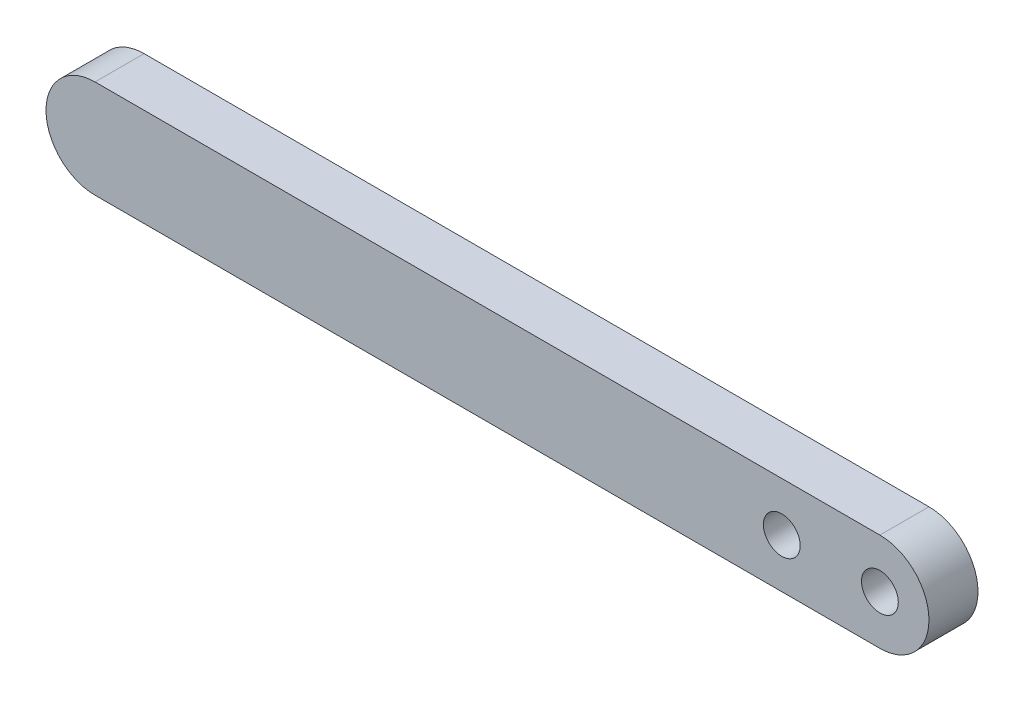
SolidWorks part; units mm, degrees
material "Plain Carbon Steel"
ref_plane "Front Plane" through (0, 0, 0) normal (0, 0, 1) x (1, 0, 0)
ref_plane "Top Plane" through (0, 0, 0) normal (0, 1, 0) x (1, 0, 0)
ref_plane "Right Plane" through (0, 0, 0) normal (1, 0, 0) x (0, 0, -1)
sketch "Handle Profile Sketch" plane through (0, 0, 0) normal (0, 0, 1) x (1, 0, 0)
  line L0 (-2.5501, 0) -> (2.5807, 0) construction
  line L1 (-2, 0) -> (2, 0) construction
  line L2 (-2, 0.25) -> (2, 0.25)
  line L3 (-2, -0.25) -> (2, -0.25)
  line L4 (1.5, 0.5151) -> (1.5, -0.9925) construction
  arc A0 (-2, 0.25) -> (-2, -0.25) centre (-2, 0) ccw
  arc A1 (2, -0.25) -> (2, 0.25) centre (2, 0) ccw
  circle A2 centre (2, 0) radius 0.0938
  circle A3 centre (1.5, 0) radius 0.0938
  point P5 (0, 0)
  dimension "D2" = 0.1875
  dimension "D3" = 0.25
  dimension "D1" = 4
  dimension "D4" = 0.5
extrude "Handle Bar Extrude" add sketch "Handle Profile Sketch" along normal mid plane 0.25
scale "Scale x25.4 to Inch Size" scale about origin uniform scaling yes scale factor 25.4
